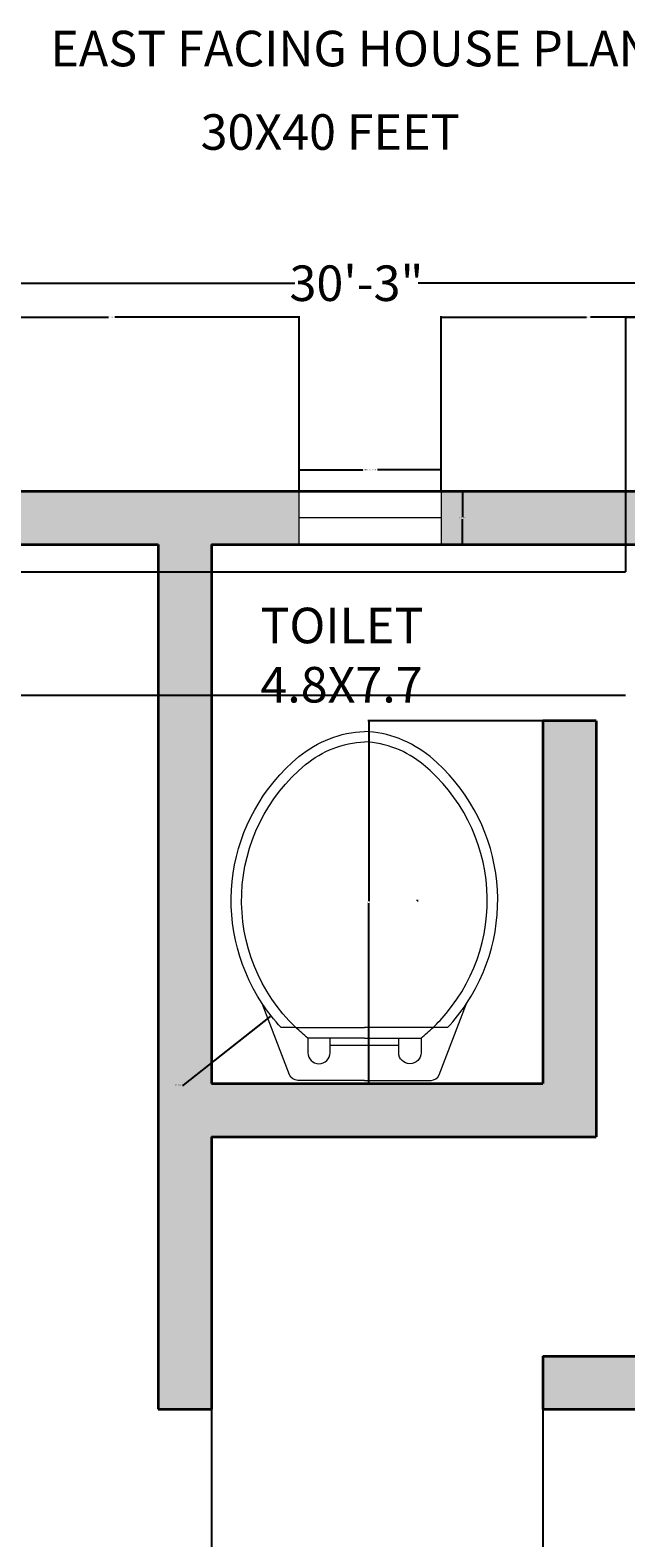
# Model space of a CAD drawing. Units: inches. Extents: x 0 to 423, y -517 to 94.
# Tile 7 of 8: x 156 to 257, y -160 to 94. Entities that reach past the tile are written whole.
import ezdxf

# ---------------------------------------------------------------- set-up
doc = ezdxf.new("R2010")
doc.units = ezdxf.units.IN
doc.header["$MEASUREMENT"] = 0
for name, color, linetype, lineweight in [('A-ANNO-DIMS', 2, 'Continuous', 18), ('A-ANNO-TEXT', 7, 'Continuous', 25), ('A-AREA-IDEN', 7, 'Continuous', 18), ('A-GLAZ', 4, 'Continuous', 18), ('A-WALL', 7, 'Continuous', 35), ('WC-Detail_dwgmodels.com', 251, 'Continuous', 13), ('WC-Outline_dwgmodels.com', 250, 'Continuous', 18)]:
    doc.layers.add(name, color=color, linetype=linetype, lineweight=lineweight)
doc.layers.add('A-WALL-PATT', color=30, linetype='Continuous', lineweight=13, true_color=0xf26722)
doc.styles.get("Standard").update_dxf_attribs({"font": 'arial.ttf'})
doc.dimstyles.get("Standard").update_dxf_attribs({"dimtxt": 0.18, "dimasz": 0.18, "dimexe": 0.18, "dimexo": 0.0625, "dimgap": 0.09, "dimtad": 0, "dimtih": 1, "dimtoh": 1, "dimdec": 0, "dimzin": 0, "dimdsep": 46, "dimlunit": 3, "dimtxsty": 'Standard', "dimcen": 0.09, "dimadec": 0, "dimazin": 0, "dimtfac": 1, "dimtdec": 0, "dimtofl": 0, "dimtmove": 0, "dimatfit": 3, "dimfxl": 1, "dimtolj": 1, "dimtzin": 0, "dimarcsym": 0})

# ---------------------------------------------------------------- blocks, each defined once
blk = doc.blocks.new('*D1')
at = {"layer": 'A-ANNO-DIMS', "color": 0, "lineweight": -2, "transparency": 16777216}
for p, q in [((29.72, 16.3), (29.72, 51.54)), ((29.9, 51.36), (200.83, 51.36)), ((392.54, 51.36), (221.62, 51.36)), ((392.72, 16.3), (392.72, 51.54))]:
    blk.add_line(p, q, dxfattribs=at)
at = {"layer": 'A-ANNO-DIMS', "color": 0, "transparency": 16777216}
for points in [[(29.9, 51.39), (29.9, 51.33), (29.72, 51.36)], [(392.54, 51.39), (392.54, 51.33), (392.72, 51.36)]]:
    blk.add_solid(points, dxfattribs=at)
at = {"layer": 'Defpoints', "color": 0, "transparency": 16777216}
for p in [(392.72, 51.36), (29.72, 16.23), (392.72, 16.23)]:
    blk.add_point(p, dxfattribs=at)
at = {"layer": 'A-ANNO-DIMS', "color": 0, "transparency": 16777216, "insert": (211.22, 51.36), "char_height": 6, "attachment_point": 5}
blk.add_mtext('\\A1;30\'-3"', dxfattribs=at)
blk = doc.blocks.new('WIN-GLAZ-24IN')
for p, q in [((0, 0), (0, 24)), ((4.5, 0), (4.5, 24)), ((9, 24), (9, 0))]:
    blk.add_line(p, q)
blk = doc.blocks.new('*D14')
at = {"layer": 'A-ANNO-DIMS', "color": 0, "lineweight": -2, "transparency": 16777216}
for p, q in [((201.52, 16.3), (201.52, 20.01)), ((201.7, 19.83), (212.29, 19.83)), ((225.34, 19.83), (214.75, 19.83)), ((225.52, 16.3), (225.52, 20.01))]:
    blk.add_line(p, q, dxfattribs=at)
at = {"layer": 'A-ANNO-DIMS', "color": 0, "transparency": 16777216}
for points in [[(201.7, 19.86), (201.7, 19.8), (201.52, 19.83)], [(225.34, 19.86), (225.34, 19.8), (225.52, 19.83)]]:
    blk.add_solid(points, dxfattribs=at)
at = {"layer": 'Defpoints', "color": 0, "transparency": 16777216}
for p in [(201.52, 19.83), (201.52, 16.23), (225.52, 16.23)]:
    blk.add_point(p, dxfattribs=at)
at = {"layer": 'A-ANNO-DIMS', "color": 0, "transparency": 16777216, "insert": (213.52, 19.83), "char_height": 0.18, "attachment_point": 5}
blk.add_mtext('\\A1;WINDOW 2\'-0" TYP.', dxfattribs=at)
blk = doc.blocks.new('*D15')
at = {"layer": 'A-ANNO-DIMS', "color": 0, "lineweight": -2, "transparency": 16777216}
for p, q in [((225.58, 16.23), (229.3, 16.23)), ((229.12, 16.05), (229.12, 11.92)), ((229.12, 7.41), (229.12, 11.55)), ((225.58, 7.23), (229.3, 7.23))]:
    blk.add_line(p, q, dxfattribs=at)
at = {"layer": 'A-ANNO-DIMS', "color": 0, "transparency": 16777216}
for points in [[(229.09, 16.05), (229.15, 16.05), (229.12, 16.23)], [(229.09, 7.41), (229.15, 7.41), (229.12, 7.23)]]:
    blk.add_solid(points, dxfattribs=at)
at = {"layer": 'Defpoints', "color": 0, "transparency": 16777216}
for p in [(225.52, 16.23), (229.12, 16.23), (225.52, 7.23)]:
    blk.add_point(p, dxfattribs=at)
at = {"layer": 'A-ANNO-DIMS', "color": 0, "transparency": 16777216, "insert": (229.12, 11.73), "char_height": 0.18, "attachment_point": 5}
blk.add_mtext('\\A1;0\'-9" TYP.', dxfattribs=at)
blk = doc.blocks.new('*D39')
at = {"layer": 'A-ANNO-DIMS', "color": 0, "lineweight": -2, "transparency": 16777216}
for p, q in [((138.22, 16.3), (138.22, 45.81)), ((138.4, 45.63), (169.33, 45.63)), ((201.34, 45.63), (170.41, 45.63)), ((201.52, 16.3), (201.52, 45.81))]:
    blk.add_line(p, q, dxfattribs=at)
at = {"layer": 'A-ANNO-DIMS', "color": 0, "transparency": 16777216}
for points in [[(138.4, 45.66), (138.4, 45.6), (138.22, 45.63)], [(201.34, 45.66), (201.34, 45.6), (201.52, 45.63)]]:
    blk.add_solid(points, dxfattribs=at)
at = {"layer": 'Defpoints', "color": 0, "transparency": 16777216}
for p in [(201.52, 45.63), (138.22, 16.23), (201.52, 16.23)]:
    blk.add_point(p, dxfattribs=at)
at = {"layer": 'A-ANNO-DIMS', "color": 0, "transparency": 16777216, "insert": (169.87, 45.63), "char_height": 0.18, "attachment_point": 5}
blk.add_mtext('\\A1;5\'-3 1/2"', dxfattribs=at)
blk = doc.blocks.new('*D40')
at = {"layer": 'A-ANNO-DIMS', "color": 0, "lineweight": -2, "transparency": 16777216}
for p, q in [((225.52, 16.3), (225.52, 45.81)), ((225.7, 45.63), (250.08, 45.63)), ((275.13, 45.63), (250.75, 45.63)), ((275.31, 16.3), (275.31, 45.81))]:
    blk.add_line(p, q, dxfattribs=at)
at = {"layer": 'A-ANNO-DIMS', "color": 0, "transparency": 16777216}
for points in [[(225.7, 45.66), (225.7, 45.6), (225.52, 45.63)], [(275.13, 45.66), (275.13, 45.6), (275.31, 45.63)]]:
    blk.add_solid(points, dxfattribs=at)
at = {"layer": 'Defpoints', "color": 0, "transparency": 16777216}
for p in [(275.31, 45.63), (225.52, 16.23), (275.31, 16.23)]:
    blk.add_point(p, dxfattribs=at)
at = {"layer": 'A-ANNO-DIMS', "color": 0, "transparency": 16777216, "insert": (250.41, 45.63), "char_height": 0.18, "attachment_point": 5}
blk.add_mtext('\\A1;4\'-2"', dxfattribs=at)
blk = doc.blocks.new('*D55')
at = {"layer": 'A-ANNO-DIMS', "color": 0, "lineweight": -2, "transparency": 16777216}
for p, q in [((242.79, -138.77), (272.3, -138.77)), ((272.12, -138.95), (272.12, -157.77)), ((272.12, -176.96), (272.12, -158.14)), ((242.79, -177.14), (272.3, -177.14))]:
    blk.add_line(p, q, dxfattribs=at)
at = {"layer": 'A-ANNO-DIMS', "color": 0, "transparency": 16777216}
for points in [[(272.09, -138.95), (272.15, -138.95), (272.12, -138.77)], [(272.09, -176.96), (272.15, -176.96), (272.12, -177.14)]]:
    blk.add_solid(points, dxfattribs=at)
at = {"layer": 'Defpoints', "color": 0, "transparency": 16777216}
for p in [(242.72, -138.77), (242.72, -177.14), (272.12, -177.14)]:
    blk.add_point(p, dxfattribs=at)
at = {"layer": 'A-ANNO-DIMS', "color": 0, "transparency": 16777216, "insert": (272.12, -157.95), "char_height": 0.18, "attachment_point": 5}
blk.add_mtext('\\A1;3\'-2 1/2"', dxfattribs=at)
blk = doc.blocks.new('*D58')
at = {"layer": 'A-ANNO-DIMS', "color": 0, "lineweight": -2, "transparency": 16777216}
for p, q in [((242.66, -22.53), (213.14, -22.53)), ((213.32, -22.71), (213.32, -52.97)), ((213.32, -83.59), (213.32, -53.33)), ((242.66, -83.77), (213.14, -83.77))]:
    blk.add_line(p, q, dxfattribs=at)
at = {"layer": 'A-ANNO-DIMS', "color": 0, "transparency": 16777216}
for points in [[(213.29, -22.71), (213.35, -22.71), (213.32, -22.53)], [(213.29, -83.59), (213.35, -83.59), (213.32, -83.77)]]:
    blk.add_solid(points, dxfattribs=at)
at = {"layer": 'Defpoints', "color": 0, "transparency": 16777216}
for p in [(213.32, -22.53), (242.72, -22.53), (242.72, -83.77)]:
    blk.add_point(p, dxfattribs=at)
at = {"layer": 'A-ANNO-DIMS', "color": 0, "transparency": 16777216, "insert": (213.32, -53.15), "char_height": 0.18, "attachment_point": 5}
blk.add_mtext('\\A1;5\'-1"', dxfattribs=at)
blk = doc.blocks.new('*D62')
at = {"layer": 'A-ANNO-DIMS', "color": 0, "lineweight": -2, "transparency": 16777216}
for p, q in [((256.72, 2.62), (256.72, 45.81)), ((256.9, 45.63), (268.86, 45.63)), ((281.49, 45.63), (269.53, 45.63)), ((281.67, 2.62), (281.67, 45.81))]:
    blk.add_line(p, q, dxfattribs=at)
at = {"layer": 'A-ANNO-DIMS', "color": 0, "transparency": 16777216}
for points in [[(256.9, 45.66), (256.9, 45.6), (256.72, 45.63)], [(281.49, 45.66), (281.49, 45.6), (281.67, 45.63)]]:
    blk.add_solid(points, dxfattribs=at)
at = {"layer": 'Defpoints', "color": 0, "transparency": 16777216}
for p in [(281.67, 45.63), (256.72, 2.55), (281.67, 2.55)]:
    blk.add_point(p, dxfattribs=at)
at = {"layer": 'A-ANNO-DIMS', "color": 0, "transparency": 16777216, "insert": (269.19, 45.63), "char_height": 0.18, "attachment_point": 5}
blk.add_mtext('\\A1;2\'-1"', dxfattribs=at)
blk = doc.blocks.new('*D63')
at = {"layer": 'A-ANNO-DIMS', "color": 0, "lineweight": -2, "transparency": 16777216}
for p, q in [((256.66, 2.55), (0.14, 2.55)), ((0.32, 2.37), (0.32, -7.66)), ((0.32, -18.06), (0.32, -8.03)), ((256.66, -18.24), (0.14, -18.24))]:
    blk.add_line(p, q, dxfattribs=at)
at = {"layer": 'A-ANNO-DIMS', "color": 0, "transparency": 16777216}
for points in [[(0.29, 2.37), (0.35, 2.37), (0.32, 2.55)], [(0.29, -18.06), (0.35, -18.06), (0.32, -18.24)]]:
    blk.add_solid(points, dxfattribs=at)
at = {"layer": 'Defpoints', "color": 0, "transparency": 16777216}
for p in [(256.72, 2.55), (0.32, -18.24), (256.72, -18.24)]:
    blk.add_point(p, dxfattribs=at)
at = {"layer": 'A-ANNO-DIMS', "color": 0, "transparency": 16777216, "insert": (0.32, -7.84), "char_height": 0.18, "attachment_point": 5}
blk.add_mtext('\\A1;1\'-9"', dxfattribs=at)
blk = doc.blocks.new('*D65')
at = {"layer": 'A-ANNO-DIMS', "color": 0, "lineweight": -2, "transparency": 16777216}
for p, q in [((186.72, -138.83), (186.72, -168.35)), ((242.72, -138.83), (242.72, -168.35)), ((186.9, -168.17), (214.39, -168.17)), ((242.54, -168.17), (215.06, -168.17))]:
    blk.add_line(p, q, dxfattribs=at)
at = {"layer": 'A-ANNO-DIMS', "color": 0, "transparency": 16777216}
for points in [[(186.9, -168.14), (186.9, -168.2), (186.72, -168.17)], [(242.54, -168.14), (242.54, -168.2), (242.72, -168.17)]]:
    blk.add_solid(points, dxfattribs=at)
at = {"layer": 'Defpoints', "color": 0, "transparency": 16777216}
for p in [(186.72, -138.77), (242.72, -138.77), (186.72, -168.17)]:
    blk.add_point(p, dxfattribs=at)
at = {"layer": 'A-ANNO-DIMS', "color": 0, "transparency": 16777216, "insert": (214.72, -168.17), "char_height": 0.18, "attachment_point": 5}
blk.add_mtext('\\A1;4\'-8"', dxfattribs=at)
blk = doc.blocks.new('*D66')
at = {"layer": 'A-ANNO-DIMS', "color": 0, "lineweight": -2, "transparency": 16777216}
for p, q in [((221.46, -52.85), (221.64, -52.85)), ((221.55, -52.94), (221.55, -52.76)), ((181.99, -84.06), (196.68, -72.47)), ((181.81, -84.06), (181.99, -84.06))]:
    blk.add_line(p, q, dxfattribs=at)
at = {"layer": 'A-ANNO-DIMS', "color": 0, "transparency": 16777216}
blk.add_solid([(196.66, -72.44), (196.7, -72.49), (196.82, -72.36)], dxfattribs=at)
at = {"layer": 'Defpoints', "color": 0, "transparency": 16777216}
for p in [(221.55, -52.85), (196.82, -72.36)]:
    blk.add_point(p, dxfattribs=at)
at = {"layer": 'A-ANNO-DIMS', "color": 0, "transparency": 16777216, "insert": (181.18, -84.06), "char_height": 0.18, "attachment_point": 5}
blk.add_mtext('\\A1;R2\'-7 1/2"', dxfattribs=at)

msp = doc.modelspace()

# ---------------------------------------------------------------- hatches: boundary and pattern name
at = {"layer": 'A-WALL-PATT'}
h = msp.add_hatch(color=256, dxfattribs=at)
h.dxf.hatch_style = 1
h.paths.add_polyline_path([(201.52, 16.23), (138.22, 16.23), (138.22, 7.23), (177.72, 7.23), (177.72, -138.77), (186.72, -138.77), (186.72, -92.77), (251.72, -92.77), (251.72, -22.53), (242.72, -22.53), (242.72, -83.77), (186.72, -83.77), (186.72, 7.23), (201.52, 7.23)])
h.paths.add_polyline_path([(78.22, 16.23), (29.72, 16.23), (29.72, -31.27), (38.72, -31.27), (38.72, 7.23), (78.22, 7.23)])
h.paths.add_polyline_path([(275.31, 16.23), (225.52, 16.23), (225.52, 7.23), (275.31, 7.23)])
h.paths.add_polyline_path([(392.72, 16.23), (335.31, 16.23), (335.31, 7.23), (383.72, 7.23), (383.72, -31.27), (392.72, -31.27)])
h.paths.add_polyline_path([(143.33, -129.77), (38.72, -129.77), (38.72, -91.27), (29.72, -91.27), (29.72, -157.27), (38.72, -157.27), (38.72, -138.77), (143.33, -138.77)])
h.paths.add_polyline_path([(186.72, -199.77), (38.72, -199.77), (38.72, -181.27), (29.72, -181.27), (29.72, -239.27), (38.72, -239.27), (38.72, -208.77), (177.72, -208.77), (177.72, -237.07), (186.72, -237.07)])
h.paths.add_polyline_path([(111.72, -161.55), (102.72, -161.55), (102.72, -199.77), (111.72, -199.77)])
h.paths.add_polyline_path([(392.72, -91.27), (383.72, -91.27), (383.72, -129.77), (242.72, -129.77), (242.72, -138.77), (383.72, -138.77), (383.72, -169.77), (392.72, -169.77)])
h.paths.add_polyline_path([(392.72, -229.77), (383.72, -229.77), (383.72, -262.77), (251.72, -262.77), (251.72, -177.14), (242.72, -177.14), (242.72, -271.77), (383.72, -271.77), (383.72, -300.77), (392.72, -300.77)])
h.paths.add_polyline_path([(392.72, -360.77), (383.72, -360.77), (383.72, -389.77), (378.42, -389.77), (378.42, -398.77), (383.72, -398.77), (383.72, -458.77), (382.72, -458.77), (382.72, -467.77), (392.72, -467.77)])
h.paths.add_polyline_path([(364.92, -389.77), (348.72, -389.77), (348.72, -467.77), (358.72, -467.77), (358.72, -458.77), (357.72, -458.77), (357.72, -398.77), (364.92, -398.77)])
h.paths.add_polyline_path([(320.72, -389.77), (283.72, -389.77), (283.72, -398.77), (320.72, -398.77)])
h.paths.add_polyline_path([(223.72, -389.77), (186.72, -389.77), (186.72, -270.38), (177.72, -270.38), (177.72, -458.77), (138.22, -458.77), (138.22, -467.77), (186.72, -467.77), (186.72, -398.77), (223.72, -398.77)])
h.paths.add_polyline_path([(143.29, -329.77), (38.72, -329.77), (38.72, -299.27), (29.72, -299.27), (29.72, -338.77), (143.29, -338.77)])
h.paths.add_polyline_path([(38.72, -374.71), (29.72, -374.71), (29.72, -398.74), (38.72, -398.74)])
h.paths.add_polyline_path([(78.22, -458.77), (38.72, -458.77), (38.72, -434.74), (29.72, -434.74), (29.72, -467.77), (78.22, -467.77)])
h.paths.add_polyline_path([(279.99, -158.17), (326.6, -158.17), (326.6, -135.78), (279.99, -135.78)], flags=25)
h.paths.add_polyline_path([(355.56, -439.13), (387, -439.13), (387, -416.66), (355.56, -416.66)], flags=9)

# ---------------------------------------------------------------- linework, layer by layer
at = {"layer": 'A-GLAZ'}
for p, q in [((201.52, 7.23), (201.52, 16.23)), ((225.52, 16.23), (225.52, 7.23))]:
    msp.add_line(p, q, dxfattribs=at)
at = {"layer": 'A-WALL'}
for p, q in [((29.72, 16.23), (392.72, 16.23)), ((38.72, 7.23), (177.72, 7.23)), ((177.72, 7.23), (177.72, -138.77)), ((186.72, 7.23), (186.72, -83.77)), ((186.72, 7.23), (383.72, 7.23)), ((242.72, -22.53), (242.72, -83.77)), ((251.72, -22.53), (242.72, -22.53)), ((251.72, -22.53), (251.72, -92.77)), ((186.72, -83.77), (242.72, -83.77)), ((186.72, -92.77), (251.72, -92.77)), ((186.72, -92.77), (186.72, -138.77)), ((242.72, -129.77), (242.72, -138.77)), ((242.72, -129.77), (383.72, -129.77)), ((177.72, -138.77), (186.72, -138.77)), ((242.72, -138.77), (383.72, -138.77))]:
    msp.add_line(p, q, dxfattribs=at)
at = {"layer": 'WC-Detail_dwgmodels.com'}
for p, q in [((200.97, -74.31), (198.5, -74.31)), ((226.62, -74.31), (224.15, -74.31))]:
    msp.add_line(p, q, dxfattribs=at)
for points in [[(198.5, -74.31, -0.040937), (195.31, -70.27, -0.163732)], [(226.62, -74.31, 0.040937), (229.81, -70.27, 0.163732)], [(203, -76.09, -0.022712), (200.97, -74.31, -0.162618)], [(212.56, -76.09), (203, -76.09, -0.476108)], [(203, -76.09), (203, -78.56, 1), (206.76, -78.56), (206.76, -77.28)], [(212.56, -76.09), (222.12, -76.09, 0.022712)], [(222.12, -76.09), (222.12, -78.56, -1), (218.36, -78.56), (218.36, -77.28)], [(222.12, -76.09, 0.022712), (224.15, -74.31, 0.162618)]]:
    msp.add_lwpolyline(points, format="xyb", dxfattribs=at)
for points in [[(206.76, -77.28), (206.76, -76.09)], [(218.36, -77.28), (218.36, -76.09)], [(206.76, -77.28), (218.36, -77.28)]]:
    msp.add_lwpolyline(points, dxfattribs=at)
at = {"layer": 'WC-Outline_dwgmodels.com'}
for p in [(200.97, -74.31), (224.15, -74.31)]:
    msp.add_line(p, (212.56, -74.31), dxfattribs=at)
for points in [[(195.31, -70.27, -0.383919), (201.49, -28.57, -0.163732), (212.56, -24.32, -0.359733)], [(229.81, -70.27, 0.383919), (223.64, -28.57, 0.163732), (212.56, -24.32, 0.359733)], [(200.97, -74.31, -0.448546), (202.61, -29.92, -0.162618), (212.56, -26.08, -0.470877)], [(225.33, -73.11, 0.431639), (222.51, -29.92, 0.162618), (212.56, -26.08, 0.470877)], [(212.56, -83.23), (201.31, -83.23, -0.31031), (199.93, -82.29), (195.31, -70.27, -0.209071)], [(212.56, -83.23), (223.81, -83.23, 0.31031), (225.19, -82.29), (229.81, -70.27, 0.209071)], [(224.15, -74.31, 0.014165), (225.33, -73.11, 0.162618)]]:
    msp.add_lwpolyline(points, format="xyb", dxfattribs=at)

# ---------------------------------------------------------------- block references
at = {"layer": 'A-GLAZ', "rotation": 89.99999999999999}
msp.add_blockref('WIN-GLAZ-24IN', (225.52, 7.24), dxfattribs=at)

# ---------------------------------------------------------------- texts
at = {"layer": 'A-ANNO-TEXT', "char_height": 6, "attachment_point": 1}
for s, insert in [('EAST FACING HOUSE PLAN', (159.5, 93.98)), ('30X40 FEET', (184.89, 79.89))]:
    msp.add_mtext(s, dxfattribs=dict(at, insert=insert))
at = {"layer": 'A-AREA-IDEN', "insert": (194.98, -3.43), "char_height": 6, "attachment_point": 1}
msp.add_mtext_dynamic_manual_height_columns('TOILET\\P4.8X7.7', width=0.5415, gutter_width=1, heights=[0], dxfattribs=at)

# ---------------------------------------------------------------- dimensions: what is measured, and where the dimension line sits
at = {"layer": 'A-ANNO-DIMS'}
for base, p1, p2, override, picture, middle in [((392.72, 51.36), (29.72, 16.23), (392.72, 16.23), {"dimtxt": 6, "dimclrd": 0, "dimclre": 0, "dimclrt": 0}, '*D1', (211.22, 51.36)), ((201.52, 45.63), (138.22, 16.23), (201.52, 16.23), {"dimdec": 1, "dimlfac": 1, "dimrnd": 0, "dimzin": 1, "dimdsep": 46, "dimlunit": 4, "dimfrac": 2}, '*D39', (169.87, 45.63)), ((275.31, 45.63), (225.52, 16.23), (275.31, 16.23), {"dimdec": 1, "dimlfac": 1, "dimrnd": 0, "dimzin": 1, "dimdsep": 46, "dimlunit": 4, "dimfrac": 2}, '*D40', (250.41, 45.63)), ((281.671, 45.6349), (256.7188, 2.5533), (281.671, 2.5533), {"dimdec": 1, "dimlfac": 1, "dimrnd": 0, "dimzin": 1, "dimdsep": 46, "dimlunit": 4, "dimfrac": 2}, '*D62', (269.1949, 45.6349))]:
    dim = msp.add_linear_dim(base=base, p1=p1, p2=p2, dimstyle='Standard', override=override, dxfattribs=at)
    dim.commit()
    dim.dimension.update_dxf_attribs({"geometry": picture, "text_midpoint": middle})
for base, p1, p2, angle, text, picture, middle in [((201.52, 19.83), (225.52, 16.23), (201.52, 16.23), 180, 'WINDOW <> TYP.', '*D14', (213.52, 19.83)), ((229.12, 16.23), (225.52, 7.23), (225.52, 16.23), 90, '<> TYP.', '*D15', (229.12, 11.73))]:
    dim = msp.add_linear_dim(base=base, p1=p1, p2=p2, angle=angle, text=text, dimstyle='Standard', override={"dimdec": 1, "dimlfac": 1, "dimrnd": 0, "dimzin": 1, "dimdsep": 46, "dimlunit": 4, "dimfrac": 2}, dxfattribs=at)
    dim.commit()
    dim.dimension.update_dxf_attribs({"geometry": picture, "text_midpoint": middle})
for base, p1, p2, angle, picture, middle in [((0.32, -18.24), (256.72, 2.55), (256.72, -18.24), 90, '*D63', (0.32, -7.84)), ((213.32, -22.53), (242.72, -83.77), (242.72, -22.53), 90, '*D58', (213.32, -53.15)), ((186.72, -168.17), (242.72, -138.77), (186.72, -138.77), 180, '*D65', (214.72, -168.17)), ((272.12, -177.14), (242.72, -138.77), (242.72, -177.14), 270, '*D55', (272.12, -157.95))]:
    dim = msp.add_linear_dim(base=base, p1=p1, p2=p2, angle=angle, dimstyle='Standard', override={"dimdec": 1, "dimlfac": 1, "dimrnd": 0, "dimzin": 1, "dimdsep": 46, "dimlunit": 4, "dimfrac": 2}, dxfattribs=at)
    dim.commit()
    dim.dimension.update_dxf_attribs({"geometry": picture, "text_midpoint": middle})
dim = msp.add_radius_dim(center=(221.55, -52.85), mpoint=(196.82, -72.36), dimstyle='Standard', override={"dimdec": 1, "dimlfac": 1, "dimrnd": 0, "dimzin": 1, "dimdsep": 46, "dimlunit": 4, "dimfrac": 2}, dxfattribs=at)
dim.commit()
dim.dimension.update_dxf_attribs({"geometry": '*D66', "text_midpoint": (181.18, -84.06), "dimtype": 164})

doc.saveas('drawing.dxf')
